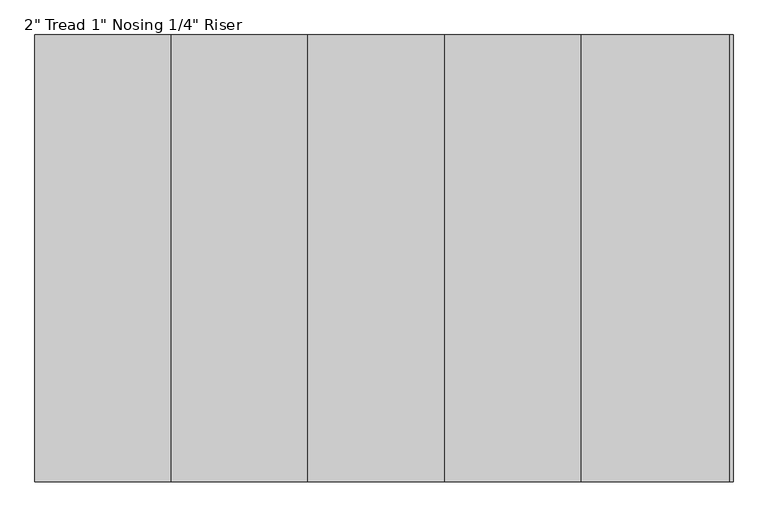
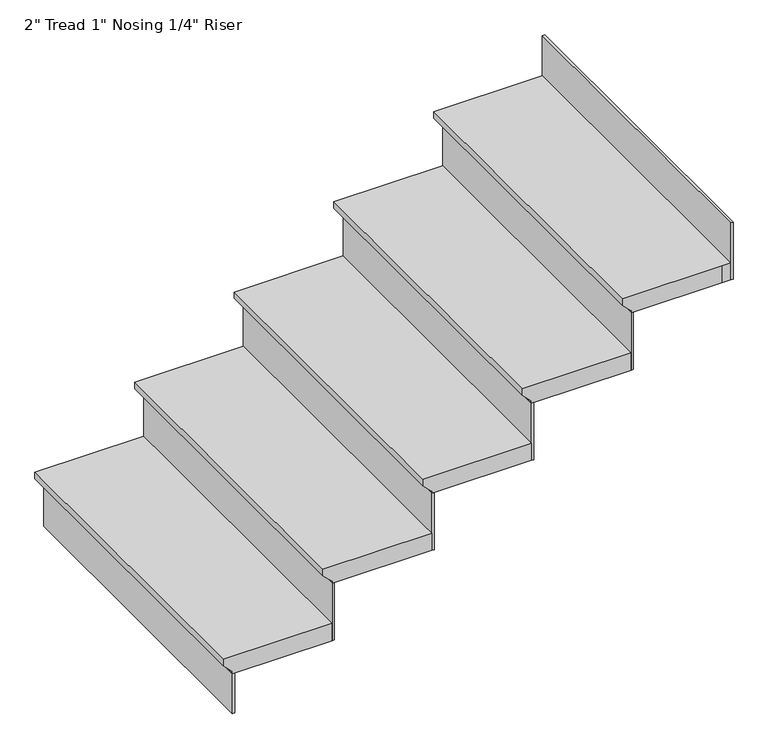
"""IFC4 building model written with IfcOpenShell, lengths in millimetres: stair flight geometry."""

from ifc_helpers import new_model, si_unit, origin, place, context, project, spatial, faceted_brep, source, transform, mapped, element, save


def stair_flight_09e20c57(model_context):
    return source(origin(), model_context, "Body", "Brep", [
        faceted_brep([(-3351.0563134, -12709.459218, 3198.2833333), (-3351.0563134, -12709.459218, 3217.3333333), (-3351.0563134, -11795.059218, 3217.3333333), (-3351.0563134, -11795.059218, 3198.2833333), (-3325.6563134, -12709.459218, 3172.8833333), (-3325.6563134, -11795.059218, 3172.8833333), (-3046.2563134, -12709.459218, 3217.3333333), (-3046.2563134, -11795.059218, 3217.3333333), (-3325.6563134, -11795.059218, 3166.5333333), (-3046.2563134, -11795.059218, 3166.5333333), (-3046.2563134, -12709.459218, 3166.5333333), (-3325.6563134, -12709.459218, 3166.5333333)], [[[0, 1, 2, 3]], [[4, 0, 3, 5]], [[2, 1, 6, 7]], [[8, 9, 10, 11]], [[2, 7, 9, 8, 5, 3]], [[8, 11, 4, 5]], [[6, 1, 0, 4, 11, 10]], [[7, 6, 10, 9]]]),
        faceted_brep([(-3325.6563134, -12709.459218, 3166.5333333), (-3325.6563134, -12709.459218, 3048.0), (-3319.3063134, -12709.459218, 3048.0), (-3319.3063134, -12709.459218, 3166.5333333), (-3325.6563134, -11795.059218, 3166.5333333), (-3319.3063134, -11795.059218, 3166.5333333), (-3319.3063134, -11795.059218, 3048.0), (-3325.6563134, -11795.059218, 3048.0)], [[[0, 1, 2, 3]], [[4, 5, 6, 7]], [[1, 0, 4, 7]], [[2, 1, 7, 6]], [[3, 2, 6, 5]], [[0, 3, 5, 4]]]),
        faceted_brep([(-3046.2563134, -12709.459218, 3335.8666667), (-3046.2563134, -12709.459218, 3166.5333333), (-3039.9063134, -12709.459218, 3166.5333333), (-3039.9063134, -12709.459218, 3335.8666667), (-3046.2563134, -11795.059218, 3335.8666667), (-3039.9063134, -11795.059218, 3335.8666667), (-3039.9063134, -11795.059218, 3166.5333333), (-3046.2563134, -11795.059218, 3166.5333333)], [[[0, 1, 2, 3]], [[4, 5, 6, 7]], [[1, 0, 4, 7]], [[2, 1, 7, 6]], [[3, 2, 6, 5]], [[0, 3, 5, 4]]]),
        faceted_brep([(-3071.6563134, -11795.059218, 3386.6666667), (-3071.6563134, -12709.459218, 3386.6666667), (-2766.8563134, -12709.459218, 3386.6666667), (-2766.8563134, -11795.059218, 3386.6666667), (-3046.2563134, -11795.059218, 3335.8666667), (-2766.8563134, -11795.059218, 3335.8666667), (-2766.8563134, -12709.459218, 3335.8666667), (-3046.2563134, -12709.459218, 3335.8666667), (-3046.2563134, -11795.059218, 3342.2166667), (-3071.6563134, -11795.059218, 3367.6166667), (-3046.2563134, -12709.459218, 3342.2166667), (-3071.6563134, -12709.459218, 3367.6166667)], [[[0, 1, 2, 3]], [[4, 5, 6, 7]], [[0, 3, 5, 4, 8, 9]], [[4, 7, 10, 8]], [[2, 1, 11, 10, 7, 6]], [[3, 2, 6, 5]], [[11, 1, 0, 9]], [[10, 11, 9, 8]]]),
        faceted_brep([(-2766.8563134, -12709.459218, 3505.2), (-2766.8563134, -12709.459218, 3335.8666667), (-2760.5063134, -12709.459218, 3335.8666667), (-2760.5063134, -12709.459218, 3505.2), (-2766.8563134, -11795.059218, 3505.2), (-2760.5063134, -11795.059218, 3505.2), (-2760.5063134, -11795.059218, 3335.8666667), (-2766.8563134, -11795.059218, 3335.8666667)], [[[0, 1, 2, 3]], [[4, 5, 6, 7]], [[1, 0, 4, 7]], [[2, 1, 7, 6]], [[3, 2, 6, 5]], [[0, 3, 5, 4]]]),
        faceted_brep([(-2792.2563134, -11795.059218, 3556.0), (-2792.2563134, -12709.459218, 3556.0), (-2487.4563134, -12709.459218, 3556.0), (-2487.4563134, -11795.059218, 3556.0), (-2766.8563134, -11795.059218, 3505.2), (-2487.4563134, -11795.059218, 3505.2), (-2487.4563134, -12709.459218, 3505.2), (-2766.8563134, -12709.459218, 3505.2), (-2766.8563134, -11795.059218, 3511.55), (-2792.2563134, -11795.059218, 3536.95), (-2766.8563134, -12709.459218, 3511.55), (-2792.2563134, -12709.459218, 3536.95)], [[[0, 1, 2, 3]], [[4, 5, 6, 7]], [[0, 3, 5, 4, 8, 9]], [[4, 7, 10, 8]], [[2, 1, 11, 10, 7, 6]], [[3, 2, 6, 5]], [[11, 1, 0, 9]], [[10, 11, 9, 8]]]),
        faceted_brep([(-2487.4563134, -12709.459218, 3674.5333333), (-2487.4563134, -12709.459218, 3505.2), (-2481.1063134, -12709.459218, 3505.2), (-2481.1063134, -12709.459218, 3674.5333333), (-2487.4563134, -11795.059218, 3674.5333333), (-2481.1063134, -11795.059218, 3674.5333333), (-2481.1063134, -11795.059218, 3505.2), (-2487.4563134, -11795.059218, 3505.2)], [[[0, 1, 2, 3]], [[4, 5, 6, 7]], [[1, 0, 4, 7]], [[2, 1, 7, 6]], [[3, 2, 6, 5]], [[0, 3, 5, 4]]]),
        faceted_brep([(-2512.8563134, -11795.059218, 3725.3333333), (-2512.8563134, -12709.459218, 3725.3333333), (-2208.0563134, -12709.459218, 3725.3333333), (-2208.0563134, -11795.059218, 3725.3333333), (-2487.4563134, -11795.059218, 3674.5333333), (-2208.0563134, -11795.059218, 3674.5333333), (-2208.0563134, -12709.459218, 3674.5333333), (-2487.4563134, -12709.459218, 3674.5333333), (-2487.4563134, -11795.059218, 3680.8833333), (-2512.8563134, -11795.059218, 3706.2833333), (-2487.4563134, -12709.459218, 3680.8833333), (-2512.8563134, -12709.459218, 3706.2833333)], [[[0, 1, 2, 3]], [[4, 5, 6, 7]], [[0, 3, 5, 4, 8, 9]], [[4, 7, 10, 8]], [[2, 1, 11, 10, 7, 6]], [[3, 2, 6, 5]], [[11, 1, 0, 9]], [[10, 11, 9, 8]]]),
        faceted_brep([(-1928.6563134, -12709.459218, 4013.2), (-1928.6563134, -12709.459218, 3843.8666667), (-1922.3063134, -12709.459218, 3843.8666667), (-1922.3063134, -12709.459218, 4013.2), (-1928.6563134, -11795.059218, 4013.2), (-1922.3063134, -11795.059218, 4013.2), (-1922.3063134, -11795.059218, 3843.8666667), (-1928.6563134, -11795.059218, 3843.8666667)], [[[0, 1, 2, 3]], [[4, 5, 6, 7]], [[1, 0, 4, 7]], [[2, 1, 7, 6]], [[3, 2, 6, 5]], [[0, 3, 5, 4]]]),
        faceted_brep([(-2208.0563134, -12709.459218, 3843.8666667), (-2208.0563134, -12709.459218, 3674.5333333), (-2201.7063134, -12709.459218, 3674.5333333), (-2201.7063134, -12709.459218, 3843.8666667), (-2208.0563134, -11795.059218, 3843.8666667), (-2201.7063134, -11795.059218, 3843.8666667), (-2201.7063134, -11795.059218, 3674.5333333), (-2208.0563134, -11795.059218, 3674.5333333)], [[[0, 1, 2, 3]], [[4, 5, 6, 7]], [[1, 0, 4, 7]], [[2, 1, 7, 6]], [[3, 2, 6, 5]], [[0, 3, 5, 4]]]),
        faceted_brep([(-1928.6563134, -11795.059218, 3894.6666667), (-1954.0563134, -11795.059218, 3894.6666667), (-2233.4563134, -11795.059218, 3894.6666667), (-2233.4563134, -12709.459218, 3894.6666667), (-1954.0563134, -12709.459218, 3894.6666667), (-1928.6563134, -12709.459218, 3894.6666667), (-1954.0563134, -11795.059218, 3843.8666667), (-1928.6563134, -11795.059218, 3843.8666667), (-1928.6563134, -12709.459218, 3843.8666667), (-1954.0563134, -12709.459218, 3843.8666667), (-2208.0563134, -12709.459218, 3843.8666667), (-2208.0563134, -11795.059218, 3843.8666667), (-2208.0563134, -11795.059218, 3850.2166667), (-2233.4563134, -11795.059218, 3875.6166667), (-2208.0563134, -12709.459218, 3850.2166667), (-2233.4563134, -12709.459218, 3875.6166667)], [[[0, 1, 2, 3, 4, 5]], [[6, 7, 8, 9, 10, 11]], [[1, 0, 7, 6]], [[2, 1, 6, 11, 12, 13]], [[11, 10, 14, 12]], [[4, 3, 15, 14, 10, 9]], [[5, 4, 9, 8]], [[0, 5, 8, 7]], [[15, 3, 2, 13]], [[14, 15, 13, 12]]]),
    ])


if __name__ == "__main__":
    model = new_model("IFC4")
    model_context = context("Model", 3, world=origin())
    ifc_project = project(units=[si_unit("LENGTHUNIT", "METRE", prefix="MILLI")], contexts=[model_context])
    site = spatial("IfcSite", under=ifc_project)
    building = spatial("IfcBuilding", under=site)
    placement = place(None, origin())
    stair_flight_shape = stair_flight_09e20c57(model_context)
    element("IfcStairFlight", 1, ObjectType="2\" Tread 1\" Nosing 1/4\" Riser", at=placement, inside=building, context=model_context, shape_type="MappedRepresentation", body=[
        mapped(stair_flight_shape, transform((0.0, 0.0, 0.0), x_axis=(1.0, 0.0, 0.0), y_axis=(0.0, 1.0, 0.0), z_axis=(0.0, 0.0, 1.0))),
    ])
    save(model, "model.ifc")
